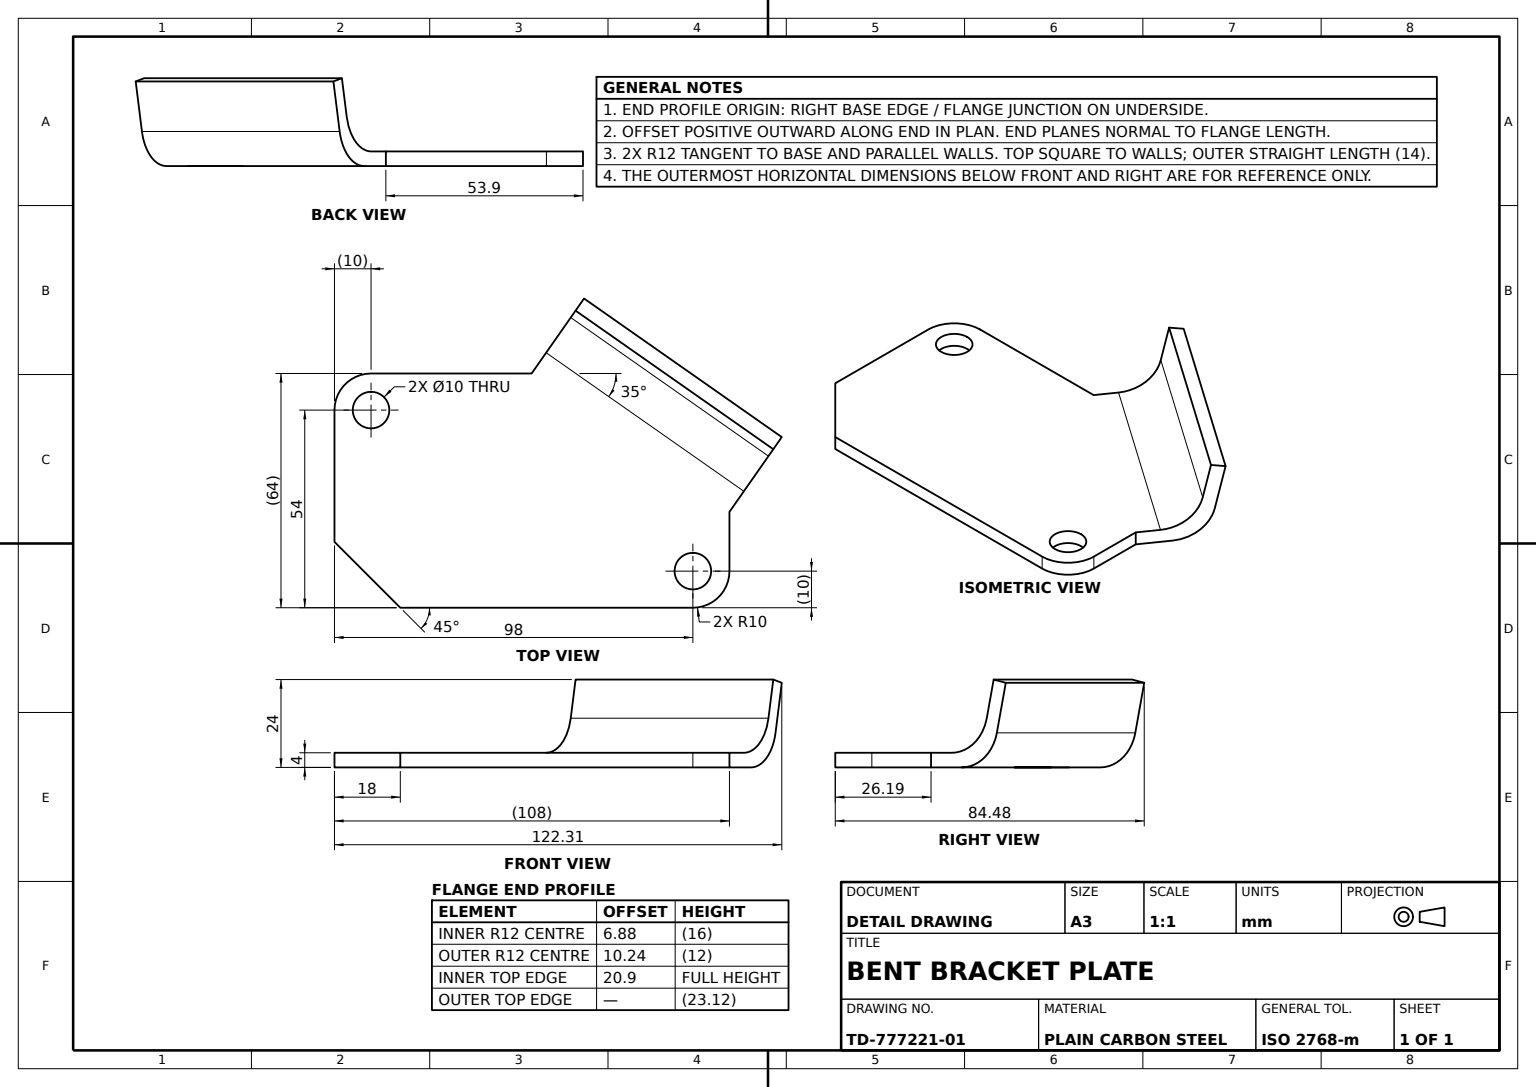
from build123d import *

# Parameters (mm, degrees)
BASE_PLATE_DEPTH             = 4
FLANGE_RISER_SKETCH_W        = 65.921827793
FLANGE_RISER_SKETCH_H        = 4
FLANGE_RISER_DEPTH           = 10
CURVED_FLANGE_DEPTH          = 66
PLATE_CORNER_FILLETS_R10_R   = 10
PLATE_CORNER_CHAMFER_18_SIZE = 18
MOUNTING_HOLES_SKETCH_R      = 5
MOUNTING_HOLES_2X_DEPTH      = 66


with BuildPart() as part:
    # Base Plate Sketch → Base Plate (new body)
    with BuildSketch(Plane(origin=(0, 0, 0), x_dir=(1, 0, 0), z_dir=(0, 1, 0))):
        Polygon((-54, -32), (54, -32), (54, -5.811207063), (0, 32), (-54, 32), align=None)
    extrude(amount=BASE_PLATE_DEPTH)

    # Flange Riser Sketch → Flange Riser (add)
    with BuildSketch(Plane(origin=(15.035081933, 0, -21.472322293), x_dir=(-0.8191520442889909, 0, -0.5735764363510474), z_dir=(0.5735764363510474, 0, -0.8191520442889909))):
        with Locations((-14.606467934, 2)):
            Rectangle(FLANGE_RISER_SKETCH_W, FLANGE_RISER_SKETCH_H)
    extrude(amount=FLANGE_RISER_DEPTH)

    # Curved Flange Profile Sketch → Curved Flange (add)
    with BuildSketch(Plane(origin=(38.964918067, 0, 27.283529357), x_dir=(0.5735764363510477, 0, -0.8191520442889908), z_dir=(0.8191520442889907, 0, 0.5735764363510476))):
        with BuildLine():
            Line((23.720397301, 4), (33.088147536, 4))
            ThreePointArc((33.088147536, 4), (40.61496291, 6.654035613), (44.812372275, 13.442158279))
            Line((44.812372275, 13.442158279), (47.116411582, 24.003044212))
            Line((47.116411582, 24.003044212), (51.162040745, 23.120420475))
            Line((51.162040745, 23.120420475), (48.17789207, 9.442158279))
            ThreePointArc((48.17789207, 9.442158279), (43.980482705, 2.654035613), (36.453667331, 0))
            Line((36.453667331, 0), (24.245794341, 0))
            Line((24.245794341, 0), (23.720397301, 4))
        make_face()
    extrude(amount=-CURVED_FLANGE_DEPTH)

    # Plate Corner Fillets R10
    plate_corner_fillets_r10_edges = [part.edges().sort_by_distance(p)[0] for p in [
        (-54, 2, -32),
        (54, 2, 32),
    ]]
    fillet(plate_corner_fillets_r10_edges, radius=PLATE_CORNER_FILLETS_R10_R)

    # Plate Corner Chamfer 18
    plate_corner_chamfer_18_edges = [part.edges().sort_by_distance(p)[0] for p in [
        (-54, 2, 32),
    ]]
    chamfer(plate_corner_chamfer_18_edges, length=PLATE_CORNER_CHAMFER_18_SIZE)

    # Mounting Holes Sketch → Mounting Holes 2x (cut)
    with BuildSketch(Plane(origin=(0, 4, 0), x_dir=(1, 0, 0), z_dir=(0, 1, 0))):
        with Locations(Location((-44, 22, 0), (0, 0, 270))):
            Circle(MOUNTING_HOLES_SKETCH_R)
        with Locations(Location((44, -22, 0), (0, 0, 270))):
            Circle(MOUNTING_HOLES_SKETCH_R)
    extrude(amount=-MOUNTING_HOLES_2X_DEPTH, mode=Mode.SUBTRACT)


solid = part.part
